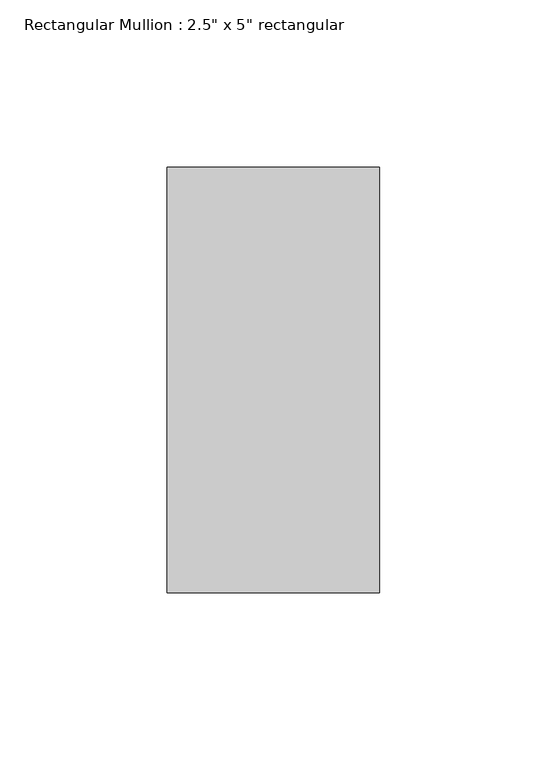
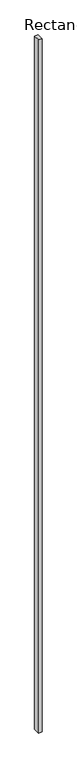
"""IFC4 building model written with IfcOpenShell, lengths in millimetres: member geometry."""

from ifc_helpers import new_model, si_unit, frame, origin, place, context, project, spatial, polyline, outline, extrude, source, transform, mapped, element, save


def member_34ed8139(model_context):
    return source(origin(), model_context, "Body", "SweptSolid", [
        extrude(outline(polyline([(0.0, 63.5), (0.0, -63.5), (-63.5, -63.5), (-63.5, 63.5), (0.0, 63.5)])), frame((0.0, 0.0, -13755.7286805), z_axis=(0.0, 0.0, 1.0), x_axis=(1.0, 0.0, 0.0)), (0.0, 0.0, 1.0), 13755.7286805),
    ])


if __name__ == "__main__":
    model = new_model("IFC4")
    model_context = context("Model", 3, world=origin())
    ifc_project = project(units=[si_unit("LENGTHUNIT", "METRE", prefix="MILLI")], contexts=[model_context])
    site = spatial("IfcSite", under=ifc_project)
    building = spatial("IfcBuilding", under=site)
    placement = place(None, origin())
    member_shape = member_34ed8139(model_context)
    element("IfcMember", 1, ObjectType="Rectangular Mullion : 2.5\" x 5\" rectangular", at=placement, inside=building, context=model_context, shape_type="MappedRepresentation", body=[
        mapped(member_shape, transform((0.0, 0.0, 0.0), x_axis=(1.0, 0.0, 0.0), y_axis=(0.0, 1.0, 0.0), z_axis=(0.0, 0.0, 1.0))),
    ])
    save(model, "model.ifc")

# Revit data of these elements
# Type "Rectangular Mullion : 2.5\" x 5\" rectangular"
#   built-in parameter 1007304 = 0.416667 (stored number, unit not read)
#   built-in parameter 1007301 = 0.104167 (stored number, unit not read)
#   built-in parameter 1007300 = 0.104167 (stored number, unit not read)
# Element 1 (IfcMember, "Rectangular Mullion : 2.5\" x 5\" rectangular")
#   Materials on its faces: "Aluminum"
# Materials
#   "Aluminum": class "Metal", colour RGB 247 247 247, transparency 0, Description = "Aluminum 6061", Cost = 0
